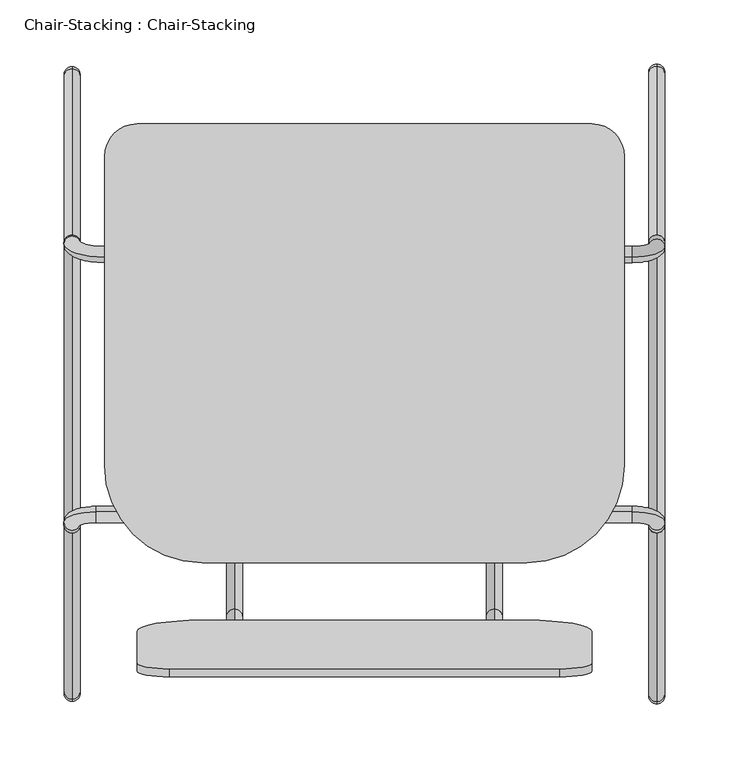
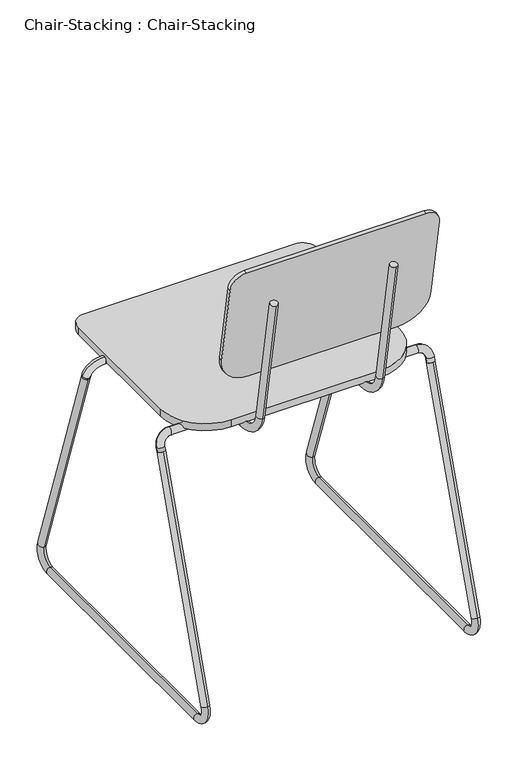
"""IFC4 building model written with IfcOpenShell, lengths in millimetres: furniture geometry, Chair-Stacking : Chair-Stacking."""

from ifc_helpers import new_model, si_unit, point, frame, frame_2d, origin, place, context, project, spatial, polyline, circle_curve, ellipse_curve, trimmed, segment, composite_curve, outline, extrude, source, transform, mapped, element, save
from ifc_brep_helpers import plane_surface, cylinder_surface, revolved_surface, advanced_brep


def chair_stacking_chair_stacking_4df0970f(model_context):
    return source(origin(), model_context, "Body", "SolidModel", [
        advanced_brep(
        [(-280.6491803, 213.2656675, 431.8), (-280.6491803, 213.2656675, 444.5), (-280.6491803, -23.0277124, 431.8), (-280.6491803, -23.0277124, 444.5), (-280.6491803, -66.802417, 481.2313385), (-280.6491803, -79.3094755, 479.0260066), (-280.6491803, -119.2282049, 705.4163709), (-280.6491803, -106.7211464, 707.6217027)],
        [
            (0, 1, circle_curve(frame((-280.6491803, 213.2656675, 438.15), z_axis=(0.0, 1.0, 0.0), x_axis=(0.0, 0.0, 1.0)), 6.35)),
            (1, 0, circle_curve(frame((-280.6491803, 213.2656675, 438.15), z_axis=(0.0, 1.0, 0.0), x_axis=(0.0, 0.0, 1.0)), 6.35)),
            (0, 2),
            (2, 3, circle_curve(frame((-280.6491803, -23.0277124, 438.15), z_axis=(0.0, 1.0, 0.0), x_axis=(0.0, 0.0, 1.0)), 6.35)),
            (3, 1),
            (3, 2, circle_curve(frame((-280.6491803, -23.0277124, 438.15), z_axis=(0.0, 1.0, 0.0), x_axis=(0.0, 0.0, 1.0)), 6.35)),
            (4, 3, circle_curve(frame((-280.6491803, -23.0277124, 488.95), z_axis=(1.0, 0.0, 0.0), x_axis=(0.0, 0.0, -1.0)), 44.45)),
            (2, 5, circle_curve(frame((-280.6491803, -23.0277124, 488.95), z_axis=(-1.0, 0.0, 0.0), x_axis=(0.0, 0.0, -1.0)), 57.15)),
            (5, 4, circle_curve(frame((-280.6491803, -73.0559463, 480.1286726), z_axis=(0.0, 0.17364817766693444, -0.9848077530122074), x_axis=(0.0, 0.9848077530122074, 0.17364817766693444)), 6.35)),
            (4, 5, circle_curve(frame((-280.6491803, -73.0559463, 480.1286726), z_axis=(0.0, 0.17364817766693444, -0.9848077530122074), x_axis=(0.0, 0.9848077530122074, 0.17364817766693444)), 6.35)),
            (6, 7, circle_curve(frame((-280.6491803, -112.9746757, 706.5190368), z_axis=(0.0, -0.1736481776669348, 0.9848077530122074), x_axis=(0.0, 0.9848077530122074, 0.1736481776669348)), 6.35)),
            (7, 6, circle_curve(frame((-280.6491803, -112.9746757, 706.5190368), z_axis=(0.0, -0.1736481776669348, 0.9848077530122074), x_axis=(0.0, 0.9848077530122074, 0.1736481776669348)), 6.35)),
            (5, 6),
            (7, 4),
        ],
        [
            plane_surface(frame((-286.9991803, 213.2656675, 438.15), z_axis=(0.0, 1.0, 0.0), x_axis=(0.0, 0.0, -1.0))),
            cylinder_surface(frame((-280.6491803, 213.2656675, 438.15), z_axis=(0.0, 1.0, 0.0), x_axis=(0.0, 0.0, 1.0)), 6.35),
            revolved_surface(trimmed(ellipse_curve(frame((-280.6491803, -23.0277124, 438.15), z_axis=(0.0, 1.0, 0.0), x_axis=(0.0, 0.0, 1.0)), 6.35, 6.35), [point((-280.6491803, -23.0277124, 431.8))], [point((-280.6491803, -23.0277124, 444.5))], True, "CARTESIAN"), (-280.6491803, -23.0277124, 488.95), (-1.0, 0.0, 0.0)),
            revolved_surface(trimmed(ellipse_curve(frame((-280.6491803, -23.0277124, 438.15), z_axis=(0.0, 1.0, 0.0), x_axis=(0.0, 0.0, 1.0)), 6.35, 6.35), [point((-280.6491803, -23.0277124, 444.5))], [point((-280.6491803, -23.0277124, 431.8))], True, "CARTESIAN"), (-280.6491803, -23.0277124, 488.95), (-1.0, 0.0, 0.0)),
            plane_surface(frame((-280.6491803, -119.2282049, 705.4163709), z_axis=(0.0, -0.17364817766692842, 0.9848077530122085), x_axis=(1.0, 0.0, 0.0))),
            cylinder_surface(frame((-280.6491803, -73.0559463, 480.1286726), z_axis=(0.0, 0.1736481776669348, -0.9848077530122074), x_axis=(0.0, 0.9848077530122074, 0.1736481776669348)), 6.35),
        ],
        [
            (0, [[1, 2]]),
            (1, [[-1, 3, 4, 5]]),
            (1, [[-2, -5, 6, -3]]),
            (2, [[7, -4, 8, 9]]),
            (3, [[-8, -6, -7, 10]]),
            (4, [[11, 12]]),
            (5, [[-9, 13, -12, 14]]),
            (5, [[-10, -14, -11, -13]]),
        ],
    ),
        advanced_brep(
        [(-77.4491803, 213.2656675, 431.8), (-77.4491803, 213.2656675, 444.5), (-77.4491803, -23.0277124, 431.8), (-77.4491803, -23.0277124, 444.5), (-77.4491803, -66.802417, 481.2313385), (-77.4491803, -79.3094755, 479.0260066), (-77.4491803, -118.9339087, 703.7473341), (-77.4491803, -106.4268502, 705.9526659)],
        [
            (0, 1, circle_curve(frame((-77.4491803, 213.2656675, 438.15), z_axis=(0.0, 1.0, 0.0), x_axis=(0.0, 0.0, 1.0)), 6.35)),
            (1, 0, circle_curve(frame((-77.4491803, 213.2656675, 438.15), z_axis=(0.0, 1.0, 0.0), x_axis=(0.0, 0.0, 1.0)), 6.35)),
            (0, 2),
            (2, 3, circle_curve(frame((-77.4491803, -23.0277124, 438.15), z_axis=(0.0, 1.0, 0.0), x_axis=(0.0, 0.0, 1.0)), 6.35)),
            (3, 1),
            (3, 2, circle_curve(frame((-77.4491803, -23.0277124, 438.15), z_axis=(0.0, 1.0, 0.0), x_axis=(0.0, 0.0, 1.0)), 6.35)),
            (4, 3, circle_curve(frame((-77.4491803, -23.0277124, 488.95), z_axis=(1.0, 0.0, 0.0), x_axis=(0.0, 0.0, -1.0)), 44.45)),
            (2, 5, circle_curve(frame((-77.4491803, -23.0277124, 488.95), z_axis=(-1.0, 0.0, 0.0), x_axis=(0.0, 0.0, -1.0)), 57.15)),
            (5, 4, circle_curve(frame((-77.4491803, -73.0559463, 480.1286726), z_axis=(0.0, 0.1736481776669385, -0.9848077530122066), x_axis=(0.0, 0.9848077530122066, 0.1736481776669385)), 6.35)),
            (4, 5, circle_curve(frame((-77.4491803, -73.0559463, 480.1286726), z_axis=(0.0, 0.1736481776669372, -0.9848077530122068), x_axis=(0.0, 0.9848077530122068, 0.1736481776669372)), 6.35)),
            (6, 7, circle_curve(frame((-77.4491803, -112.6803794, 704.85), z_axis=(0.0, -0.17364817766693896, 0.9848077530122066), x_axis=(0.0, 0.9848077530122066, 0.17364817766693896)), 6.35)),
            (7, 6, circle_curve(frame((-77.4491803, -112.6803794, 704.85), z_axis=(0.0, -0.17364817766693896, 0.9848077530122066), x_axis=(0.0, 0.9848077530122066, 0.17364817766693896)), 6.35)),
            (5, 6),
            (7, 4),
        ],
        [
            plane_surface(frame((-83.7991803, 213.2656675, 438.15), z_axis=(0.0, 1.0, 0.0), x_axis=(0.0, 0.0, -1.0))),
            cylinder_surface(frame((-77.4491803, 213.2656675, 438.15), z_axis=(0.0, 1.0, 0.0), x_axis=(0.0, 0.0, 1.0)), 6.35),
            revolved_surface(trimmed(ellipse_curve(frame((-77.4491803, -23.0277124, 438.15), z_axis=(0.0, 1.0, 0.0), x_axis=(0.0, 0.0, 1.0)), 6.35, 6.35), [point((-77.4491803, -23.0277124, 431.8))], [point((-77.4491803, -23.0277124, 444.5))], True, "CARTESIAN"), (-77.4491803, -23.0277124, 488.95), (-1.0, 0.0, 0.0)),
            revolved_surface(trimmed(ellipse_curve(frame((-77.4491803, -23.0277124, 438.15), z_axis=(0.0, 1.0, 0.0), x_axis=(0.0, 0.0, 1.0)), 6.35, 6.35), [point((-77.4491803, -23.0277124, 444.5))], [point((-77.4491803, -23.0277124, 431.8))], True, "CARTESIAN"), (-77.4491803, -23.0277124, 488.95), (-1.0, 0.0, 0.0)),
            plane_surface(frame((-77.4491803, -118.9339087, 703.7473341), z_axis=(0.0, -0.17364817766692892, 0.9848077530122084), x_axis=(1.0, 0.0, 0.0))),
            cylinder_surface(frame((-77.4491803, -73.0559463, 480.1286726), z_axis=(0.0, 0.17364817766693896, -0.9848077530122066), x_axis=(0.0, 0.9848077530122066, 0.17364817766693896)), 6.35),
        ],
        [
            (0, [[1, 2]]),
            (1, [[-1, 3, 4, 5]]),
            (1, [[-2, -5, 6, -3]]),
            (2, [[7, -4, 8, 9]]),
            (3, [[-8, -6, -7, 10]]),
            (4, [[11, 12]]),
            (5, [[-9, 13, -12, 14]]),
            (5, [[-10, -14, -11, -13]]),
        ],
    ),
        extrude(outline(composite_curve([segment(trimmed(circle_curve(frame_2d((-1.2491803, 286.7314636)), 25.4), [point((-1.2491803, 312.1314636))], [point((24.1508197, 286.7314636))], False, "CARTESIAN"), True, "CONTINUOUS"), segment(polyline([(24.1508197, 286.7314636), (24.1508197, 45.4314636)]), True, "CONTINUOUS"), segment(trimmed(circle_curve(frame_2d((-52.0491803, 45.4314636)), 76.2), [point((24.1508197, 45.4314636))], [point((-52.0491803, -30.7685364))], False, "CARTESIAN"), True, "CONTINUOUS"), segment(polyline([(-52.0491803, -30.7685364), (-306.0491803, -30.7685364)]), True, "CONTINUOUS"), segment(trimmed(circle_curve(frame_2d((-306.0491803, 45.4314636)), 76.2), [point((-306.0491803, -30.7685364))], [point((-382.2491803, 45.4314636))], False, "CARTESIAN"), True, "CONTINUOUS"), segment(polyline([(-382.2491803, 45.4314636), (-382.2491803, 286.7314636)]), True, "CONTINUOUS"), segment(trimmed(circle_curve(frame_2d((-356.8491803, 286.7314636)), 25.4), [point((-382.2491803, 286.7314636))], [point((-356.8491803, 312.1314636))], False, "CARTESIAN"), True, "CONTINUOUS"), segment(polyline([(-356.8491803, 312.1314636), (-1.2491803, 312.1314636)]), True, "CONTINUOUS")], self_intersect=False)), frame((0.0, 0.0, 444.5), z_axis=(0.0, 0.0, 1.0), x_axis=(1.0, 0.0, 0.0)), (0.0, 0.0, 1.0), 12.7),
        extrude(outline(composite_curve([segment(polyline([(-304.8, 0.0), (0.0, 0.0)]), True, "CONTINUOUS"), segment(trimmed(circle_curve(frame_2d((0.0, -25.4)), 25.4), [point((0.0, 0.0))], [point((25.4, -25.4))], False, "CARTESIAN"), True, "CONTINUOUS"), segment(polyline([(25.4, -25.4), (25.4, -168.3013626)]), True, "CONTINUOUS"), segment(trimmed(circle_curve(frame_2d((-25.4, -168.3013626)), 50.8), [point((25.4, -168.3013626))], [point((-25.4, -219.1013626))], False, "CARTESIAN"), True, "CONTINUOUS"), segment(polyline([(-25.4, -219.1013626), (-279.4, -219.1013626)]), True, "CONTINUOUS"), segment(trimmed(circle_curve(frame_2d((-279.4, -168.3013626)), 50.8), [point((-279.4, -219.1013626))], [point((-330.2, -168.3013626))], False, "CARTESIAN"), True, "CONTINUOUS"), segment(polyline([(-330.2, -168.3013626), (-330.2, -25.4)]), True, "CONTINUOUS"), segment(trimmed(circle_curve(frame_2d((-304.8, -25.4)), 25.4), [point((-330.2, -25.4))], [point((-304.8, 0.0))], False, "CARTESIAN"), True, "CONTINUOUS")], self_intersect=False)), frame((-331.4491803, -119.9531376, 782.6640535), z_axis=(0.0, 0.9848077530122084, 0.17364817766692858), x_axis=(-1.0, 0.0, 0.0)), (0.0, 0.0, 1.0), 6.35),
        advanced_brep(
        [(55.9008197, 219.2327758, 419.1211728), (43.2008197, 219.2327758, 419.1211728), (55.9008197, 216.3017292, 427.6700586), (43.2008197, 216.3017292, 427.6700586), (30.5008197, 212.1828103, 439.6835721), (30.5008197, 208.0638914, 451.6970857), (-382.2491803, 208.0638914, 451.6970857), (-382.2491803, 212.1828103, 439.6835721), (-401.2991803, 218.3611887, 421.6633019), (-413.9991803, 218.3611887, 421.6633019), (-413.9991803, 219.2424531, 419.0929473), (-401.2991803, 219.2424531, 419.0929473)],
        [
            (0, 1, circle_curve(frame((49.5508197, 219.2327758, 419.1211728), z_axis=(0.0, 0.32432432432432967, -0.9459459459459442), x_axis=(-1.0, 0.0, 0.0)), 6.35)),
            (1, 0, circle_curve(frame((49.5508197, 219.2327758, 419.1211728), z_axis=(0.0, 0.32432432432432967, -0.9459459459459442), x_axis=(-1.0, 0.0, 0.0)), 6.35)),
            (0, 2),
            (2, 3, circle_curve(frame((49.5508197, 216.3017292, 427.6700586), z_axis=(0.0, 0.32432432432432967, -0.9459459459459442), x_axis=(-1.0, 0.0, 0.0)), 6.35)),
            (3, 1),
            (3, 2, circle_curve(frame((49.5508197, 216.3017292, 427.6700586), z_axis=(0.0, 0.32432432432432967, -0.9459459459459442), x_axis=(-1.0, 0.0, 0.0)), 6.35)),
            (4, 3, circle_curve(frame((30.5008197, 216.3017292, 427.6700586), z_axis=(0.0, 0.9459459459459447, 0.3243243243243281), x_axis=(1.0, 0.0, 0.0)), 12.7)),
            (2, 5, circle_curve(frame((30.5008197, 216.3017292, 427.6700586), z_axis=(0.0, -0.9459459459459447, -0.3243243243243281), x_axis=(1.0, 0.0, 0.0)), 25.4)),
            (5, 4, circle_curve(frame((30.5008197, 210.1233509, 445.6903289), z_axis=(1.0, 0.0, 0.0), x_axis=(0.0, 0.32432432432432745, -0.9459459459459449)), 6.35)),
            (4, 5, circle_curve(frame((30.5008197, 210.1233509, 445.6903289), z_axis=(1.0, 0.0, 0.0), x_axis=(0.0, 0.32432432432432745, -0.9459459459459449)), 6.35)),
            (5, 6),
            (6, 7, circle_curve(frame((-382.2491803, 210.1233509, 445.6903289), z_axis=(1.0, 0.0, 0.0), x_axis=(0.0, 0.32432432432432745, -0.9459459459459449)), 6.35)),
            (7, 4),
            (7, 6, circle_curve(frame((-382.2491803, 210.1233509, 445.6903289), z_axis=(1.0, 0.0, 0.0), x_axis=(0.0, 0.32432432432432745, -0.9459459459459449)), 6.35)),
            (8, 7, circle_curve(frame((-382.2491803, 218.3611887, 421.6633019), z_axis=(0.0, 0.9459459459459447, 0.3243243243243281), x_axis=(0.0, -0.3243243243243281, 0.9459459459459447)), 19.05)),
            (6, 9, circle_curve(frame((-382.2491803, 218.3611887, 421.6633019), z_axis=(0.0, -0.9459459459459447, -0.3243243243243281), x_axis=(0.0, -0.3243243243243281, 0.9459459459459447)), 31.75)),
            (9, 8, circle_curve(frame((-407.6491803, 218.3611887, 421.6633019), z_axis=(0.0, -0.324324324324328, 0.9459459459459447), x_axis=(1.0000000000000002, 0.0, 0.0)), 6.35)),
            (8, 9, circle_curve(frame((-407.6491803, 218.3611887, 421.6633019), z_axis=(0.0, -0.324324324324328, 0.9459459459459447), x_axis=(1.0000000000000002, 0.0, 0.0)), 6.35)),
            (10, 11, circle_curve(frame((-407.6491803, 219.2424531, 419.0929473), z_axis=(0.0, 0.32432432432432784, -0.9459459459459449), x_axis=(1.0, 0.0, 0.0)), 6.35)),
            (11, 10, circle_curve(frame((-407.6491803, 219.2424531, 419.0929473), z_axis=(0.0, 0.32432432432432784, -0.9459459459459449), x_axis=(1.0, 0.0, 0.0)), 6.35)),
            (9, 10),
            (11, 8),
        ],
        [
            plane_surface(frame((49.5508197, 213.226019, 417.0617133), z_axis=(0.0, 0.32432432432433117, -0.9459459459459437), x_axis=(1.0, 0.0, 0.0))),
            cylinder_surface(frame((49.5508197, 219.2327758, 419.1211728), z_axis=(0.0, 0.32432432432432967, -0.9459459459459442), x_axis=(-1.0, 0.0, 0.0)), 6.35),
            revolved_surface(trimmed(ellipse_curve(frame((49.5508197, 216.3017292, 427.6700586), z_axis=(0.0, 0.32432432432432823, -0.9459459459459447), x_axis=(-1.0, 0.0, 0.0)), 6.35, 6.35), [point((55.9008197, 216.3017292, 427.6700586))], [point((43.2008197, 216.3017292, 427.6700586))], True, "CARTESIAN"), (30.5008197, 216.3017292, 427.6700586), (0.0, -0.9459459459459447, -0.3243243243243281)),
            revolved_surface(trimmed(ellipse_curve(frame((49.5508197, 216.3017292, 427.6700586), z_axis=(0.0, 0.32432432432432823, -0.9459459459459447), x_axis=(-1.0, 0.0, 0.0)), 6.35, 6.35), [point((43.2008197, 216.3017292, 427.6700586))], [point((55.9008197, 216.3017292, 427.6700586))], True, "CARTESIAN"), (30.5008197, 216.3017292, 427.6700586), (0.0, -0.9459459459459447, -0.3243243243243281)),
            cylinder_surface(frame((30.5008197, 210.1233509, 445.6903289), z_axis=(1.0, 0.0, 0.0), x_axis=(0.0, 0.32432432432432745, -0.9459459459459449)), 6.35),
            revolved_surface(trimmed(ellipse_curve(frame((-382.2491803, 210.1233509, 445.6903289), z_axis=(1.0000000000000002, 0.0, 0.0), x_axis=(0.0, 0.3243243243243276, -0.9459459459459449)), 6.35, 6.35), [point((-382.2491803, 208.0638914, 451.6970857))], [point((-382.2491803, 212.1828103, 439.6835721))], True, "CARTESIAN"), (-382.2491803, 218.3611887, 421.6633019), (0.0, -0.9459459459459447, -0.3243243243243281)),
            revolved_surface(trimmed(ellipse_curve(frame((-382.2491803, 210.1233509, 445.6903289), z_axis=(1.0000000000000002, 0.0, 0.0), x_axis=(0.0, 0.3243243243243276, -0.9459459459459449)), 6.35, 6.35), [point((-382.2491803, 212.1828103, 439.6835721))], [point((-382.2491803, 208.0638914, 451.6970857))], True, "CARTESIAN"), (-382.2491803, 218.3611887, 421.6633019), (0.0, -0.9459459459459447, -0.3243243243243281)),
            plane_surface(frame((-407.6491803, 225.2492099, 421.1524068), z_axis=(0.0, 0.3243243243243264, -0.9459459459459453), x_axis=(1.0, 0.0, 0.0))),
            cylinder_surface(frame((-407.6491803, 218.3611887, 421.6633019), z_axis=(0.0, -0.3243243243243278, 0.9459459459459447), x_axis=(1.0, 0.0, 0.0)), 6.35),
        ],
        [
            (0, [[1, 2]]),
            (1, [[-1, 3, 4, 5]]),
            (1, [[-2, -5, 6, -3]]),
            (2, [[7, -4, 8, 9]]),
            (3, [[-8, -6, -7, 10]]),
            (4, [[-9, 11, 12, 13]]),
            (4, [[-10, -13, 14, -11]]),
            (5, [[15, -12, 16, 17]]),
            (6, [[-16, -14, -15, 18]]),
            (7, [[19, 20]]),
            (8, [[-17, 21, -20, 22]]),
            (8, [[-18, -22, -19, -21]]),
        ],
    ),
        advanced_brep(
        [(55.9008197, -1.3812406, 419.0879461), (43.2008197, -1.3812406, 419.0879461), (55.9008197, 0.7944914, 425.4338312), (43.2008197, 0.7944914, 425.4338312), (30.5008197, 4.9134104, 437.4473447), (30.5008197, 9.0323293, 449.4608582), (-388.5991803, 9.0323293, 449.4608582), (-388.5991803, 4.9134104, 437.4473447), (-401.2991803, 0.7944914, 425.4338312), (-413.9991803, 0.7944914, 425.4338312), (-413.9991803, -1.3997864, 419.0338542), (-401.2991803, -1.3997864, 419.0338542)],
        [
            (0, 1, circle_curve(frame((49.5508197, -1.3812406, 419.0879461), z_axis=(0.0, -0.32432432432432495, -0.9459459459459457), x_axis=(-1.0, 0.0, 0.0)), 6.35)),
            (1, 0, circle_curve(frame((49.5508197, -1.3812406, 419.0879461), z_axis=(0.0, -0.32432432432432495, -0.9459459459459457), x_axis=(-1.0, 0.0, 0.0)), 6.35)),
            (0, 2),
            (2, 3, circle_curve(frame((49.5508197, 0.7944914, 425.4338312), z_axis=(0.0, -0.32432432432432495, -0.9459459459459457), x_axis=(-1.0, 0.0, 0.0)), 6.35)),
            (3, 1),
            (3, 2, circle_curve(frame((49.5508197, 0.7944914, 425.4338312), z_axis=(0.0, -0.32432432432432495, -0.9459459459459457), x_axis=(-1.0, 0.0, 0.0)), 6.35)),
            (4, 3, circle_curve(frame((30.5008197, 0.7944914, 425.4338312), z_axis=(0.0, 0.9459459459459458, -0.3243243243243246), x_axis=(1.0, 0.0, 0.0)), 12.7)),
            (2, 5, circle_curve(frame((30.5008197, 0.7944914, 425.4338312), z_axis=(0.0, -0.9459459459459458, 0.3243243243243246), x_axis=(1.0, 0.0, 0.0)), 25.4)),
            (5, 4, circle_curve(frame((30.5008197, 6.9728698, 443.4541014), z_axis=(1.0, 0.0, 0.0), x_axis=(0.0, -0.3243243243243236, -0.9459459459459462)), 6.35)),
            (4, 5, circle_curve(frame((30.5008197, 6.9728698, 443.4541014), z_axis=(1.0, 0.0, 0.0), x_axis=(0.0, -0.3243243243243236, -0.9459459459459462)), 6.35)),
            (5, 6),
            (6, 7, circle_curve(frame((-388.5991803, 6.9728698, 443.4541014), z_axis=(1.0, 0.0, 0.0), x_axis=(0.0, -0.3243243243243236, -0.9459459459459462)), 6.35)),
            (7, 4),
            (7, 6, circle_curve(frame((-388.5991803, 6.9728698, 443.4541014), z_axis=(1.0, 0.0, 0.0), x_axis=(0.0, -0.3243243243243236, -0.9459459459459462)), 6.35)),
            (8, 7, circle_curve(frame((-388.5991803, 0.7944914, 425.4338312), z_axis=(0.0, 0.9459459459459458, -0.3243243243243246), x_axis=(0.0, 0.3243243243243246, 0.9459459459459458)), 12.7)),
            (6, 9, circle_curve(frame((-388.5991803, 0.7944914, 425.4338312), z_axis=(0.0, -0.9459459459459458, 0.3243243243243246), x_axis=(0.0, 0.3243243243243246, 0.9459459459459458)), 25.4)),
            (9, 8, circle_curve(frame((-407.6491803, 0.7944914, 425.4338312), z_axis=(0.0, 0.3243243243243247, 0.9459459459459458), x_axis=(1.0, 0.0, 0.0)), 6.35)),
            (8, 9, circle_curve(frame((-407.6491803, 0.7944914, 425.4338312), z_axis=(0.0, 0.3243243243243247, 0.9459459459459458), x_axis=(1.0, 0.0, 0.0)), 6.35)),
            (10, 11, circle_curve(frame((-407.6491803, -1.3997864, 419.0338542), z_axis=(0.0, -0.3243243243243242, -0.945945945945946), x_axis=(1.0, 0.0, 0.0)), 6.35)),
            (11, 10, circle_curve(frame((-407.6491803, -1.3997864, 419.0338542), z_axis=(0.0, -0.3243243243243242, -0.945945945945946), x_axis=(1.0, 0.0, 0.0)), 6.35)),
            (9, 10),
            (11, 8),
        ],
        [
            plane_surface(frame((49.5508197, -7.3879973, 421.1474055), z_axis=(0.0, -0.32432432432432273, -0.9459459459459466), x_axis=(1.0, 0.0, 0.0))),
            cylinder_surface(frame((49.5508197, -1.3812406, 419.0879461), z_axis=(0.0, -0.32432432432432495, -0.9459459459459457), x_axis=(-1.0, 0.0, 0.0)), 6.35),
            revolved_surface(trimmed(ellipse_curve(frame((49.5508197, 0.7944914, 425.4338312), z_axis=(0.0, -0.32432432432432456, -0.9459459459459458), x_axis=(-1.0, 0.0, 0.0)), 6.35, 6.35), [point((55.9008197, 0.7944914, 425.4338312))], [point((43.2008197, 0.7944914, 425.4338312))], True, "CARTESIAN"), (30.5008197, 0.7944914, 425.4338312), (0.0, -0.9459459459459458, 0.3243243243243246)),
            revolved_surface(trimmed(ellipse_curve(frame((49.5508197, 0.7944914, 425.4338312), z_axis=(0.0, -0.32432432432432456, -0.9459459459459458), x_axis=(-1.0, 0.0, 0.0)), 6.35, 6.35), [point((43.2008197, 0.7944914, 425.4338312))], [point((55.9008197, 0.7944914, 425.4338312))], True, "CARTESIAN"), (30.5008197, 0.7944914, 425.4338312), (0.0, -0.9459459459459458, 0.3243243243243246)),
            cylinder_surface(frame((30.5008197, 6.9728698, 443.4541014), z_axis=(1.0, 0.0, 0.0), x_axis=(0.0, -0.3243243243243236, -0.9459459459459462)), 6.35),
            revolved_surface(trimmed(ellipse_curve(frame((-388.5991803, 6.9728698, 443.4541014), z_axis=(1.0, 0.0, 0.0), x_axis=(0.0, -0.3243243243243236, -0.9459459459459462)), 6.35, 6.35), [point((-388.5991803, 9.0323293, 449.4608582))], [point((-388.5991803, 4.9134104, 437.4473447))], True, "CARTESIAN"), (-388.5991803, 0.7944914, 425.4338312), (0.0, -0.9459459459459458, 0.3243243243243246)),
            revolved_surface(trimmed(ellipse_curve(frame((-388.5991803, 6.9728698, 443.4541014), z_axis=(1.0, 0.0, 0.0), x_axis=(0.0, -0.3243243243243236, -0.9459459459459462)), 6.35, 6.35), [point((-388.5991803, 4.9134104, 437.4473447))], [point((-388.5991803, 9.0323293, 449.4608582))], True, "CARTESIAN"), (-388.5991803, 0.7944914, 425.4338312), (0.0, -0.9459459459459458, 0.3243243243243246)),
            plane_surface(frame((-407.6491803, 4.6069704, 416.9743947), z_axis=(0.0, -0.3243243243243226, -0.9459459459459466), x_axis=(1.0, 0.0, 0.0))),
            cylinder_surface(frame((-407.6491803, 0.7944914, 425.4338312), z_axis=(0.0, 0.3243243243243242, 0.945945945945946), x_axis=(1.0, 0.0, 0.0)), 6.35),
        ],
        [
            (0, [[1, 2]]),
            (1, [[-1, 3, 4, 5]]),
            (1, [[-2, -5, 6, -3]]),
            (2, [[7, -4, 8, 9]]),
            (3, [[-8, -6, -7, 10]]),
            (4, [[-9, 11, 12, 13]]),
            (4, [[-10, -13, 14, -11]]),
            (5, [[15, -12, 16, 17]]),
            (6, [[-16, -14, -15, 18]]),
            (7, [[19, 20]]),
            (8, [[-17, 21, -20, 22]]),
            (8, [[-18, -22, -19, -21]]),
        ],
    ),
        advanced_brep(
        [(-407.6491803, 225.2492099, 421.1524068), (-407.6491803, 213.2356963, 417.0334879), (-407.6491803, 355.2281045, 42.0472973), (-407.6491803, 343.214591, 37.9283784), (-407.6491803, 325.1943208, 12.7), (-407.6491803, 325.1943208, 0.0), (-407.6491803, -107.3313935, 0.0), (-407.6491803, -107.3313935, 12.7), (-407.6491803, -125.3516638, 37.9283784), (-407.6491803, -137.3651773, 42.0472973), (-407.6491803, -7.4065431, 421.0933136), (-407.6491803, 4.6069704, 416.9743947)],
        [
            (0, 1, circle_curve(frame((-407.6491803, 219.2424531, 419.0929473), z_axis=(0.0, -0.3243243243243311, 0.9459459459459437), x_axis=(0.0, -0.9459459459459437, -0.3243243243243311)), 6.35)),
            (1, 0, circle_curve(frame((-407.6491803, 219.2424531, 419.0929473), z_axis=(0.0, -0.3243243243243311, 0.9459459459459437), x_axis=(0.0, -0.9459459459459437, -0.3243243243243311)), 6.35)),
            (0, 2),
            (2, 3, circle_curve(frame((-407.6491803, 349.2213478, 39.9878378), z_axis=(0.0, -0.3243243243243311, 0.9459459459459437), x_axis=(0.0, -0.9459459459459437, -0.3243243243243311)), 6.35)),
            (3, 1),
            (3, 2, circle_curve(frame((-407.6491803, 349.2213478, 39.9878378), z_axis=(0.0, -0.3243243243243311, 0.9459459459459437), x_axis=(0.0, -0.9459459459459437, -0.3243243243243311)), 6.35)),
            (4, 3, circle_curve(frame((-407.6491803, 325.1943208, 31.75), z_axis=(1.0, 0.0, 0.0), x_axis=(0.0, 0.9459459459459434, 0.3243243243243317)), 19.05)),
            (2, 5, circle_curve(frame((-407.6491803, 325.1943208, 31.75), z_axis=(-1.0, 0.0, 0.0), x_axis=(0.0, 0.9459459459459434, 0.3243243243243317)), 31.75)),
            (5, 4, circle_curve(frame((-407.6491803, 325.1943208, 6.35), z_axis=(0.0, 1.0, 0.0), x_axis=(0.0, 0.0, 1.0)), 6.35)),
            (4, 5, circle_curve(frame((-407.6491803, 325.1943208, 6.35), z_axis=(0.0, 0.9999999999999999, 0.0), x_axis=(0.0, 0.0, 0.9999999999999999)), 6.35)),
            (5, 6),
            (6, 7, circle_curve(frame((-407.6491803, -107.3313935, 6.35), z_axis=(0.0, 1.0, 0.0), x_axis=(0.0, 0.0, 1.0)), 6.35)),
            (7, 4),
            (7, 6, circle_curve(frame((-407.6491803, -107.3313935, 6.35), z_axis=(0.0, 1.0, 0.0), x_axis=(0.0, 0.0, 1.0)), 6.35)),
            (8, 7, circle_curve(frame((-407.6491803, -107.3313935, 31.75), z_axis=(1.0, 0.0, 0.0), x_axis=(0.0, 0.0, -1.0)), 19.05)),
            (6, 9, circle_curve(frame((-407.6491803, -107.3313935, 31.75), z_axis=(-1.0, 0.0, 0.0), x_axis=(0.0, 0.0, -1.0)), 31.75)),
            (9, 8, circle_curve(frame((-407.6491803, -131.3584206, 39.9878378), z_axis=(0.0, -0.3243243243243189, -0.9459459459459478), x_axis=(0.0, 0.9459459459459478, -0.3243243243243189)), 6.35)),
            (8, 9, circle_curve(frame((-407.6491803, -131.3584206, 39.9878378), z_axis=(0.0, -0.3243243243243206, -0.9459459459459473), x_axis=(0.0, 0.9459459459459473, -0.3243243243243206)), 6.35)),
            (10, 11, circle_curve(frame((-407.6491803, -1.3997864, 419.0338542), z_axis=(0.0, 0.3243243243243217, 0.9459459459459468), x_axis=(0.0, 0.9459459459459468, -0.3243243243243217)), 6.35)),
            (11, 10, circle_curve(frame((-407.6491803, -1.3997864, 419.0338542), z_axis=(0.0, 0.3243243243243217, 0.9459459459459468), x_axis=(0.0, 0.9459459459459468, -0.3243243243243217)), 6.35)),
            (9, 10),
            (11, 8),
        ],
        [
            plane_surface(frame((-407.6491803, 225.2492099, 421.1524068), z_axis=(0.0, -0.32432432432432773, 0.9459459459459448), x_axis=(1.0, 0.0, 0.0))),
            cylinder_surface(frame((-407.6491803, 219.2424531, 419.0929473), z_axis=(0.0, -0.3243243243243311, 0.9459459459459437), x_axis=(0.0, -0.9459459459459437, -0.3243243243243311)), 6.35),
            revolved_surface(trimmed(ellipse_curve(frame((-407.6491803, 349.2213478, 39.9878378), z_axis=(0.0, -0.3243243243243347, 0.9459459459459424), x_axis=(0.0, -0.9459459459459424, -0.3243243243243347)), 6.35, 6.35), [point((-407.6491803, 355.2281045, 42.0472973))], [point((-407.6491803, 343.214591, 37.9283784))], True, "CARTESIAN"), (-407.6491803, 325.1943208, 31.75), (-1.0, 0.0, 0.0)),
            revolved_surface(trimmed(ellipse_curve(frame((-407.6491803, 349.2213478, 39.9878378), z_axis=(0.0, -0.3243243243243347, 0.9459459459459424), x_axis=(0.0, -0.9459459459459424, -0.3243243243243347)), 6.35, 6.35), [point((-407.6491803, 343.214591, 37.9283784))], [point((-407.6491803, 355.2281045, 42.0472973))], True, "CARTESIAN"), (-407.6491803, 325.1943208, 31.75), (-1.0, 0.0, 0.0)),
            cylinder_surface(frame((-407.6491803, 325.1943208, 6.35), z_axis=(0.0, 1.0, 0.0), x_axis=(0.0, 0.0, 1.0)), 6.35),
            revolved_surface(trimmed(ellipse_curve(frame((-407.6491803, -107.3313935, 6.35), z_axis=(0.0, 1.0, 0.0), x_axis=(0.0, 0.0, 1.0)), 6.35, 6.35), [point((-407.6491803, -107.3313935, 0.0))], [point((-407.6491803, -107.3313935, 12.7))], True, "CARTESIAN"), (-407.6491803, -107.3313935, 31.75), (-1.0, 0.0, 0.0)),
            revolved_surface(trimmed(ellipse_curve(frame((-407.6491803, -107.3313935, 6.35), z_axis=(0.0, 1.0, 0.0), x_axis=(0.0, 0.0, 1.0)), 6.35, 6.35), [point((-407.6491803, -107.3313935, 12.7))], [point((-407.6491803, -107.3313935, 0.0))], True, "CARTESIAN"), (-407.6491803, -107.3313935, 31.75), (-1.0, 0.0, 0.0)),
            plane_surface(frame((-407.6491803, -7.4065431, 421.0933136), z_axis=(0.0, 0.324324324324323, 0.9459459459459465), x_axis=(1.0, 0.0, 0.0))),
            cylinder_surface(frame((-407.6491803, -131.3584206, 39.9878378), z_axis=(0.0, -0.3243243243243217, -0.9459459459459468), x_axis=(0.0, 0.9459459459459468, -0.3243243243243217)), 6.35),
        ],
        [
            (0, [[1, 2]]),
            (1, [[-1, 3, 4, 5]]),
            (1, [[-2, -5, 6, -3]]),
            (2, [[7, -4, 8, 9]]),
            (3, [[-8, -6, -7, 10]]),
            (4, [[-9, 11, 12, 13]]),
            (4, [[-10, -13, 14, -11]]),
            (5, [[15, -12, 16, 17]]),
            (6, [[-16, -14, -15, 18]]),
            (7, [[19, 20]]),
            (8, [[-17, 21, -20, 22]]),
            (8, [[-18, -22, -19, -21]]),
        ],
    ),
        advanced_brep(
        [(49.5508197, 225.2597598, 421.1875673), (49.5508197, 213.2656675, 417.0124327), (49.5508197, 357.1892841, 42.1878365), (49.5508197, 345.1951918, 38.0127019), (49.5508197, 327.2040533, 12.7), (49.5508197, 327.2040533, 0.0), (49.5508197, -109.3411268, 0.0), (49.5508197, -109.3411268, 12.7), (49.5508197, -127.3337908, 38.0083179), (49.5508197, -139.3289001, 42.1805298), (49.5508197, -7.5008737, 421.186106), (49.5508197, 4.4942357, 417.013894)],
        [
            (0, 1, circle_curve(frame((49.5508197, 219.2627136, 419.1), z_axis=(0.0, -0.3287507573582007, 0.9444167192168982), x_axis=(0.0, -0.9444167192168982, -0.3287507573582007)), 6.35)),
            (1, 0, circle_curve(frame((49.5508197, 219.2627136, 419.1), z_axis=(0.0, -0.3287507573582007, 0.9444167192168982), x_axis=(0.0, -0.9444167192168982, -0.3287507573582007)), 6.35)),
            (0, 2),
            (2, 3, circle_curve(frame((49.5508197, 351.1922379, 40.1002692), z_axis=(0.0, -0.3287507573582007, 0.9444167192168982), x_axis=(0.0, -0.9444167192168982, -0.3287507573582007)), 6.35)),
            (3, 1),
            (3, 2, circle_curve(frame((49.5508197, 351.1922379, 40.1002692), z_axis=(0.0, -0.3287507573582007, 0.9444167192168982), x_axis=(0.0, -0.9444167192168982, -0.3287507573582007)), 6.35)),
            (4, 3, circle_curve(frame((49.5508197, 327.2040533, 31.75), z_axis=(1.0, 0.0, 0.0), x_axis=(0.0, 0.944416719216897, 0.3287507573582041)), 19.05)),
            (2, 5, circle_curve(frame((49.5508197, 327.2040533, 31.75), z_axis=(-1.0, 0.0, 0.0), x_axis=(0.0, 0.944416719216897, 0.3287507573582041)), 31.75)),
            (5, 4, circle_curve(frame((49.5508197, 327.2040533, 6.35), z_axis=(0.0, 1.0, 0.0), x_axis=(0.0, 0.0, 1.0)), 6.35)),
            (4, 5, circle_curve(frame((49.5508197, 327.2040533, 6.35), z_axis=(0.0, 0.9999999999999999, 0.0), x_axis=(0.0, 0.0, 0.9999999999999999)), 6.35)),
            (5, 6),
            (6, 7, circle_curve(frame((49.5508197, -109.3411268, 6.35), z_axis=(0.0, 1.0, 0.0), x_axis=(0.0, 0.0, 1.0)), 6.35)),
            (7, 4),
            (7, 6, circle_curve(frame((49.5508197, -109.3411268, 6.35), z_axis=(0.0, 1.0, 0.0), x_axis=(0.0, 0.0, 1.0)), 6.35)),
            (8, 7, circle_curve(frame((49.5508197, -109.3411268, 31.75), z_axis=(1.0, 0.0, 0.0), x_axis=(0.0, 0.0, -1.0)), 19.05)),
            (6, 9, circle_curve(frame((49.5508197, -109.3411268, 31.75), z_axis=(-1.0, 0.0, 0.0), x_axis=(0.0, 0.0, -1.0)), 31.75)),
            (9, 8, circle_curve(frame((49.5508197, -133.3313455, 40.0944239), z_axis=(0.0, -0.3285206249412718, -0.9444967967061594), x_axis=(0.0, 0.9444967967061594, -0.3285206249412718)), 6.35)),
            (8, 9, circle_curve(frame((49.5508197, -133.3313455, 40.0944239), z_axis=(0.0, -0.3285206249412754, -0.9444967967061582), x_axis=(0.0, 0.9444967967061582, -0.3285206249412754)), 6.35)),
            (10, 11, circle_curve(frame((49.5508197, -1.503319, 419.1), z_axis=(0.0, 0.3285206249412728, 0.9444967967061592), x_axis=(0.0, 0.9444967967061592, -0.3285206249412728)), 6.35)),
            (11, 10, circle_curve(frame((49.5508197, -1.503319, 419.1), z_axis=(0.0, 0.3285206249412728, 0.9444967967061592), x_axis=(0.0, 0.9444967967061592, -0.3285206249412728)), 6.35)),
            (9, 10),
            (11, 8),
        ],
        [
            plane_surface(frame((49.5508197, 225.2597598, 421.1875673), z_axis=(0.0, -0.3287507573582023, 0.9444167192168977), x_axis=(1.0, 0.0, 0.0))),
            cylinder_surface(frame((49.5508197, 219.2627136, 419.1), z_axis=(0.0, -0.3287507573582007, 0.9444167192168982), x_axis=(0.0, -0.9444167192168982, -0.3287507573582007)), 6.35),
            revolved_surface(trimmed(ellipse_curve(frame((49.5508197, 351.1922379, 40.1002692), z_axis=(0.0, -0.32875075735820414, 0.944416719216897), x_axis=(0.0, -0.944416719216897, -0.32875075735820414)), 6.35, 6.35), [point((49.5508197, 357.1892841, 42.1878365))], [point((49.5508197, 345.1951918, 38.0127019))], True, "CARTESIAN"), (49.5508197, 327.2040533, 31.75), (-1.0, 0.0, 0.0)),
            revolved_surface(trimmed(ellipse_curve(frame((49.5508197, 351.1922379, 40.1002692), z_axis=(0.0, -0.32875075735820414, 0.944416719216897), x_axis=(0.0, -0.944416719216897, -0.32875075735820414)), 6.35, 6.35), [point((49.5508197, 345.1951918, 38.0127019))], [point((49.5508197, 357.1892841, 42.1878365))], True, "CARTESIAN"), (49.5508197, 327.2040533, 31.75), (-1.0, 0.0, 0.0)),
            cylinder_surface(frame((49.5508197, 327.2040533, 6.35), z_axis=(0.0, 1.0, 0.0), x_axis=(0.0, 0.0, 1.0)), 6.35),
            revolved_surface(trimmed(ellipse_curve(frame((49.5508197, -109.3411268, 6.35), z_axis=(0.0, 1.0, 0.0), x_axis=(0.0, 0.0, 1.0)), 6.35, 6.35), [point((49.5508197, -109.3411268, 0.0))], [point((49.5508197, -109.3411268, 12.7))], True, "CARTESIAN"), (49.5508197, -109.3411268, 31.75), (-1.0, 0.0, 0.0)),
            revolved_surface(trimmed(ellipse_curve(frame((49.5508197, -109.3411268, 6.35), z_axis=(0.0, 1.0, 0.0), x_axis=(0.0, 0.0, 1.0)), 6.35, 6.35), [point((49.5508197, -109.3411268, 12.7))], [point((49.5508197, -109.3411268, 0.0))], True, "CARTESIAN"), (49.5508197, -109.3411268, 31.75), (-1.0, 0.0, 0.0)),
            plane_surface(frame((49.5508197, -7.5008737, 421.186106), z_axis=(0.0, 0.3285206249412714, 0.9444967967061596), x_axis=(1.0, 0.0, 0.0))),
            cylinder_surface(frame((49.5508197, -133.3313455, 40.0944239), z_axis=(0.0, -0.3285206249412728, -0.9444967967061592), x_axis=(0.0, 0.9444967967061592, -0.3285206249412728)), 6.35),
        ],
        [
            (0, [[1, 2]]),
            (1, [[-1, 3, 4, 5]]),
            (1, [[-2, -5, 6, -3]]),
            (2, [[7, -4, 8, 9]]),
            (3, [[-8, -6, -7, 10]]),
            (4, [[-9, 11, 12, 13]]),
            (4, [[-10, -13, 14, -11]]),
            (5, [[15, -12, 16, 17]]),
            (6, [[-16, -14, -15, 18]]),
            (7, [[19, 20]]),
            (8, [[-17, 21, -20, 22]]),
            (8, [[-18, -22, -19, -21]]),
        ],
    ),
    ])


if __name__ == "__main__":
    model = new_model("IFC4")
    model_context = context("Model", 3, world=origin())
    ifc_project = project(units=[si_unit("LENGTHUNIT", "METRE", prefix="MILLI")], contexts=[model_context])
    site = spatial("IfcSite", under=ifc_project)
    building = spatial("IfcBuilding", under=site)
    placement = place(None, origin())
    chair_stacking_chair_stacking_shape = chair_stacking_chair_stacking_4df0970f(model_context)
    element("IfcFurniture", 1, ObjectType="Chair-Stacking : Chair-Stacking", at=placement, inside=building, context=model_context, shape_type="MappedRepresentation", body=[
        mapped(chair_stacking_chair_stacking_shape, transform((0.0, 0.0, 0.0), x_axis=(1.0, 0.0, 0.0), y_axis=(0.0, 1.0, 0.0), z_axis=(0.0, 0.0, 1.0))),
    ])
    save(model, "model.ifc")

# Revit data of these elements
# Type "Chair-Stacking : Chair-Stacking"
#   Assembly Code = "E2020200"
#   Seat/Back Material = Cherry
#   Default Elevation = 0
# Element 1 (IfcFurniture, "Chair-Stacking : Chair-Stacking")
#   Materials on its faces: "Steel, Chrome Plated", "Cherry"
# Materials
#   "Cherry": class "Wood", colour RGB 226 177 128, transparency 0, Description = "Prunus Serotina", Cost = 0
#   "Steel, Chrome Plated": class "Metal", colour RGB 17 17 17, transparency 0, Description = "Chromiuim plated steel", Cost = 0
